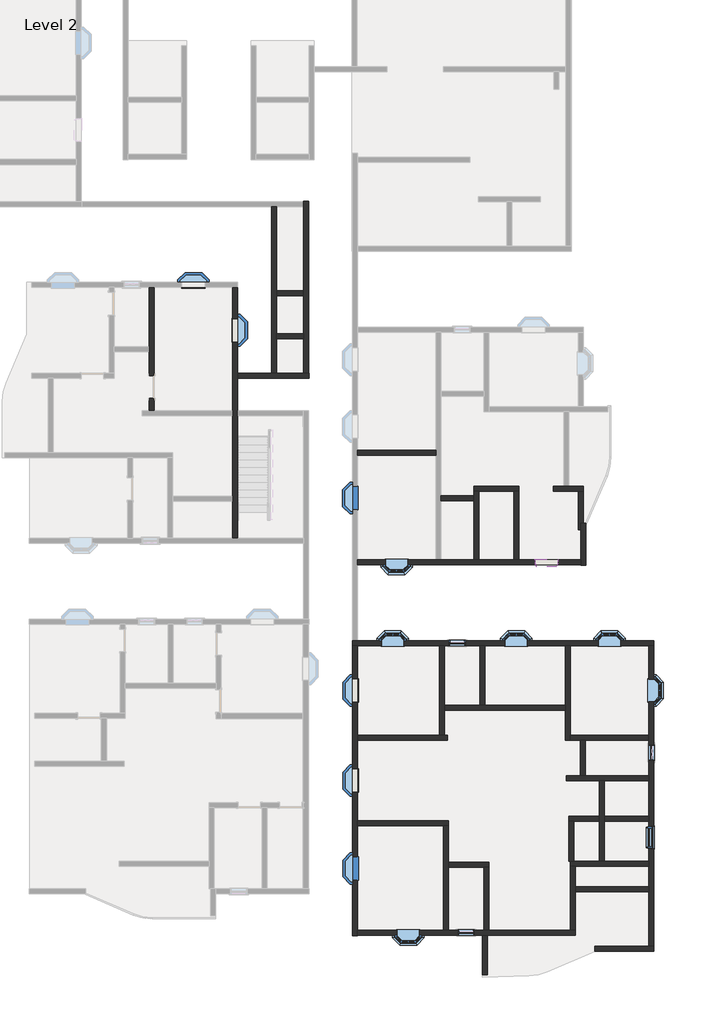
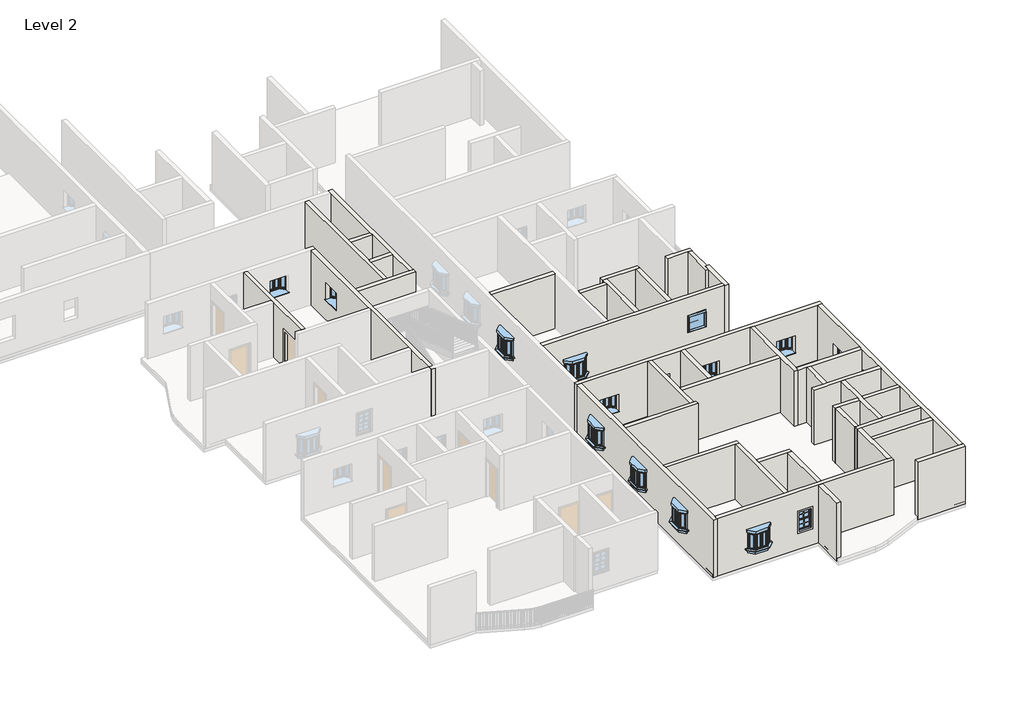
# One storey, part 2 of 14: 40 walls, 17 windows.
"""IFC4 building model written with IfcOpenShell, lengths in millimetres."""

from ifc_helpers import new_model, si_unit, frame, origin, place, context, project, spatial, polyline, outline, extrude, faceted_brep, transform, mapped, element, save
from components import window_910x910mm_67ef725a, window_8debb0fa, windows_sgl_w_glazing_bars_910x910mm_256712d0

model = new_model("IFC4")

# Units and contexts
model_context = context("Model", 3, world=origin())
ifc_project = project(units=[si_unit("LENGTHUNIT", "METRE", prefix="MILLI")], contexts=[model_context])

# Site, building, storey
site = spatial("IfcSite", under=ifc_project)
building = spatial("IfcBuilding", under=site)
storey = spatial("IfcBuildingStorey", under=building, Name="Level 2", Elevation=3048.0)

# Walls
placement = place(None, origin())
element("IfcWall", 1, ObjectType="4.5\" p", at=placement, inside=storey, context=model_context, shape_type="SweptSolid", body=[
    extrude(outline(polyline([(6070.4380523, -28382.7374148), (6070.4380523, -26796.6042694), (6273.6380523, -26796.6042694), (6273.6380523, -28382.7374148), (6070.4380523, -28382.7374148)])), frame((0.0, 0.0, 3048.0), z_axis=(0.0, 0.0, 1.0), x_axis=(1.0, 0.0, 0.0)), (0.0, 0.0, 1.0), 3048.0),
])
element("IfcWall", 2, ObjectType="4.5\" p", at=placement, inside=storey, context=model_context, shape_type="Brep", body=[
    faceted_brep([(10639.6896214, -27431.6042694, 3048.0), (13030.0380523, -27431.6042694, 3048.0), (13030.0380523, -27431.6042694, 6096.0), (10639.6896214, -27431.6042694, 6096.0), (10639.6896214, -27228.4042694, 3048.0), (10639.6896214, -27228.4042694, 6096.0), (12814.1380523, -27228.4042694, 6096.0), (13017.3380523, -27228.4042694, 6096.0), (13030.0380523, -27228.4042694, 6096.0), (13030.0380523, -27228.4042694, 3048.0), (13017.3380523, -27228.4042694, 3048.0), (12814.1380523, -27228.4042694, 3048.0)], [[[0, 1, 2, 3]], [[4, 5, 6, 7, 8, 9, 10, 11]], [[1, 0, 4, 11, 10, 9]], [[2, 1, 9, 8]], [[3, 2, 8, 7, 6, 5]], [[0, 3, 5, 4]]]),
])
element("IfcWall", 3, ObjectType="4.5\" p", at=placement, inside=storey, context=model_context, shape_type="Brep", body=[
    faceted_brep([(1015.8380523, -18878.1542694, 3048.0), (4648.0380523, -18878.1542694, 3048.0), (4648.0380523, -18878.1542694, 6096.0), (1015.8380523, -18878.1542694, 6096.0), (1015.8380523, -18674.9542694, 3048.0), (1015.8380523, -18674.9542694, 6096.0), (4336.8880523, -18674.9542694, 6096.0), (4540.0880523, -18674.9542694, 6096.0), (4648.0380523, -18674.9542694, 6096.0), (4648.0380523, -18674.9542694, 3048.0), (4540.0880523, -18674.9542694, 3048.0), (4336.8880523, -18674.9542694, 3048.0)], [[[0, 1, 2, 3]], [[4, 5, 6, 7, 8, 9, 10, 11]], [[1, 0, 4, 11, 10, 9]], [[2, 1, 9, 8]], [[3, 2, 8, 7, 6, 5]], [[0, 3, 5, 4]]]),
])
element("IfcWall", 4, ObjectType="4.5\" p", at=placement, inside=storey, context=model_context, shape_type="Brep", body=[
    faceted_brep([(4336.8880523, -15049.1042694, 3048.0), (4336.8880523, -18674.9542694, 3048.0), (4336.8880523, -18674.9542694, 6096.0), (4336.8880523, -15049.1042694, 6096.0), (4540.0880523, -15049.1042694, 3048.0), (4540.0880523, -15049.1042694, 6096.0), (4540.0880523, -17455.7542694, 6096.0), (4540.0880523, -17658.9542694, 6096.0), (4540.0880523, -18674.9542694, 6096.0), (4540.0880523, -18674.9542694, 3048.0), (4540.0880523, -17658.9542694, 3048.0), (4540.0880523, -17455.7542694, 3048.0)], [[[0, 1, 2, 3]], [[4, 5, 6, 7, 8, 9, 10, 11]], [[1, 0, 4, 11, 10, 9]], [[3, 2, 8, 7, 6, 5]], [[0, 3, 5, 4]], [[2, 1, 9, 8]]]),
])
element("IfcWall", 5, ObjectType="4.5\" p", at=placement, inside=storey, context=model_context, shape_type="Brep", body=[
    faceted_brep([(4540.0880523, -17658.9542694, 3048.0), (9442.2880523, -17658.9542694, 3048.0), (9442.2880523, -17658.9542694, 6096.0), (4540.0880523, -17658.9542694, 6096.0), (4540.0880523, -17455.7542694, 3048.0), (4540.0880523, -17455.7542694, 6096.0), (5975.1880523, -17455.7542694, 6096.0), (6178.3880523, -17455.7542694, 6096.0), (9442.2880523, -17455.7542694, 6096.0), (9442.2880523, -17455.7542694, 3048.0), (6178.3880523, -17455.7542694, 3048.0), (5975.1880523, -17455.7542694, 3048.0)], [[[0, 1, 2, 3]], [[4, 5, 6, 7, 8, 9, 10, 11]], [[1, 0, 4, 11, 10, 9]], [[3, 2, 8, 7, 6, 5]], [[0, 3, 5, 4]], [[2, 1, 9, 8]]]),
])
element("IfcWall", 6, ObjectType="4.5\" p", at=placement, inside=storey, context=model_context, shape_type="SweptSolid", body=[
    extrude(outline(polyline([(5975.1880523, -17455.7542694), (5975.1880523, -15049.1042694), (6178.3880523, -15049.1042694), (6178.3880523, -17455.7542694), (5975.1880523, -17455.7542694)])), frame((0.0, 0.0, 3048.0), z_axis=(0.0, 0.0, 1.0), x_axis=(1.0, 0.0, 0.0)), (0.0, 0.0, 1.0), 3048.0),
])
element("IfcWall", 7, ObjectType="4.5\" p", at=placement, inside=storey, context=model_context, shape_type="Brep", body=[
    faceted_brep([(9442.2880523, -15049.1042694, 3048.0), (9442.2880523, -17455.7542694, 3048.0), (9442.2880523, -17658.9542694, 3048.0), (9442.2880523, -18871.8042694, 3048.0), (9442.2880523, -18871.8042694, 6096.0), (9442.2880523, -17658.9542694, 6096.0), (9442.2880523, -17455.7542694, 6096.0), (9442.2880523, -15049.1042694, 6096.0), (9645.4880523, -15049.1042694, 3048.0), (9645.4880523, -15049.1042694, 6096.0), (9645.4880523, -18668.6042694, 6096.0), (9645.4880523, -18871.8042694, 6096.0), (9645.4880523, -18871.8042694, 3048.0), (9645.4880523, -18668.6042694, 3048.0)], [[[0, 1, 2, 3, 4, 5, 6, 7]], [[8, 9, 10, 11, 12, 13]], [[3, 2, 1, 0, 8, 13, 12]], [[7, 6, 5, 4, 11, 10, 9]], [[0, 7, 9, 8]], [[4, 3, 12, 11]]]),
])
element("IfcWall", 8, ObjectType="4.5\" p", at=placement, inside=storey, context=model_context, shape_type="Brep", body=[
    faceted_brep([(1015.8380523, -22345.2542694, 3048.0), (4489.2880523, -22345.2542694, 3048.0), (4692.4880523, -22345.2542694, 3048.0), (4692.4880523, -22345.2542694, 6096.0), (4489.2880523, -22345.2542694, 6096.0), (1015.8380523, -22345.2542694, 6096.0), (1015.8380523, -22142.0542694, 3048.0), (1015.8380523, -22142.0542694, 6096.0), (4692.4880523, -22142.0542694, 6096.0), (4692.4880523, -22142.0542694, 3048.0)], [[[0, 1, 2, 3, 4, 5]], [[6, 7, 8, 9]], [[2, 1, 0, 6, 9]], [[5, 4, 3, 8, 7]], [[0, 5, 7, 6]], [[3, 2, 9, 8]]]),
])
element("IfcWall", 9, ObjectType="4.5\" p", at=placement, inside=storey, context=model_context, shape_type="Brep", body=[
    faceted_brep([(4489.2880523, -22345.2542694, 3048.0), (4489.2880523, -26580.7042694, 3048.0), (4489.2880523, -26580.7042694, 6096.0), (4489.2880523, -22345.2542694, 6096.0), (4692.4880523, -22345.2542694, 3048.0), (4692.4880523, -22345.2542694, 6096.0), (4692.4880523, -23818.4542694, 6096.0), (4692.4880523, -24021.6542694, 6096.0), (4692.4880523, -26580.7042694, 6096.0), (4692.4880523, -26580.7042694, 3048.0), (4692.4880523, -24021.6542694, 3048.0), (4692.4880523, -23818.4542694, 3048.0)], [[[0, 1, 2, 3]], [[4, 5, 6, 7, 8, 9, 10, 11]], [[1, 0, 4, 11, 10, 9]], [[3, 2, 8, 7, 6, 5]], [[0, 3, 5, 4]], [[2, 1, 9, 8]]]),
])
element("IfcWall", 10, ObjectType="4.5\" p", at=placement, inside=storey, context=model_context, shape_type="Brep", body=[
    faceted_brep([(4692.4880523, -24021.6542694, 3048.0), (6127.5880523, -24021.6542694, 3048.0), (6330.7880523, -24021.6542694, 3048.0), (6330.7880523, -24021.6542694, 6096.0), (6127.5880523, -24021.6542694, 6096.0), (4692.4880523, -24021.6542694, 6096.0), (4692.4880523, -23818.4542694, 3048.0), (4692.4880523, -23818.4542694, 6096.0), (6330.7880523, -23818.4542694, 6096.0), (6330.7880523, -23818.4542694, 3048.0)], [[[0, 1, 2, 3, 4, 5]], [[6, 7, 8, 9]], [[2, 1, 0, 6, 9]], [[5, 4, 3, 8, 7]], [[0, 5, 7, 6]], [[3, 2, 9, 8]]]),
])
element("IfcWall", 11, ObjectType="4.5\" p", at=placement, inside=storey, context=model_context, shape_type="SweptSolid", body=[
    extrude(outline(polyline([(6127.5880523, -26580.7042694), (6127.5880523, -24021.6542694), (6330.7880523, -24021.6542694), (6330.7880523, -26580.7042694), (6127.5880523, -26580.7042694)])), frame((0.0, 0.0, 3048.0), z_axis=(0.0, 0.0, 1.0), x_axis=(1.0, 0.0, 0.0)), (0.0, 0.0, 1.0), 3048.0),
])
element("IfcWall", 12, ObjectType="4.5\" p", at=placement, inside=storey, context=model_context, shape_type="Brep", body=[
    faceted_brep([(9645.4880523, -18871.8042694, 3048.0), (10051.8880523, -18871.8042694, 3048.0), (10255.0880523, -18871.8042694, 3048.0), (12814.1380523, -18871.8042694, 3048.0), (12814.1380523, -18871.8042694, 6096.0), (10255.0880523, -18871.8042694, 6096.0), (10051.8880523, -18871.8042694, 6096.0), (9645.4880523, -18871.8042694, 6096.0), (9645.4880523, -18668.6042694, 3048.0), (9645.4880523, -18668.6042694, 6096.0), (12814.1380523, -18668.6042694, 6096.0), (12814.1380523, -18668.6042694, 3048.0)], [[[0, 1, 2, 3, 4, 5, 6, 7]], [[8, 9, 10, 11]], [[3, 2, 1, 0, 8, 11]], [[7, 6, 5, 4, 10, 9]], [[0, 7, 9, 8]], [[4, 3, 11, 10]]]),
])
element("IfcWall", 13, ObjectType="4.5\" p", at=placement, inside=storey, context=model_context, shape_type="SweptSolid", body=[
    extrude(outline(polyline([(10051.8880523, -20313.2542694), (10051.8880523, -18871.8042694), (10255.0880523, -18871.8042694), (10255.0880523, -20313.2542694), (10051.8880523, -20313.2542694)])), frame((0.0, 0.0, 3048.0), z_axis=(0.0, 0.0, 1.0), x_axis=(1.0, 0.0, 0.0)), (0.0, 0.0, 1.0), 3048.0),
])
element("IfcWall", 14, ObjectType="4.5\" p", at=placement, inside=storey, context=model_context, shape_type="Brep", body=[
    faceted_brep([(12814.1380523, -20313.2542694, 3048.0), (10255.0880523, -20313.2542694, 3048.0), (10051.8880523, -20313.2542694, 3048.0), (9486.7380523, -20313.2542694, 3048.0), (9486.7380523, -20313.2542694, 6096.0), (10051.8880523, -20313.2542694, 6096.0), (10255.0880523, -20313.2542694, 6096.0), (12814.1380523, -20313.2542694, 6096.0), (12814.1380523, -20516.4542694, 3048.0), (12814.1380523, -20516.4542694, 6096.0), (11017.0880523, -20516.4542694, 6096.0), (10813.8880523, -20516.4542694, 6096.0), (9486.7380523, -20516.4542694, 6096.0), (9486.7380523, -20516.4542694, 3048.0), (10813.8880523, -20516.4542694, 3048.0), (11017.0880523, -20516.4542694, 3048.0)], [[[0, 1, 2, 3, 4, 5, 6, 7]], [[8, 9, 10, 11, 12, 13, 14, 15]], [[3, 2, 1, 0, 8, 15, 14, 13]], [[4, 3, 13, 12]], [[7, 6, 5, 4, 12, 11, 10, 9]], [[0, 7, 9, 8]]]),
])
element("IfcWall", 15, ObjectType="4.5\" p", at=placement, inside=storey, context=model_context, shape_type="Brep", body=[
    faceted_brep([(10813.8880523, -20516.4542694, 3048.0), (10813.8880523, -21951.5542694, 3048.0), (10813.8880523, -22154.7542694, 3048.0), (10813.8880523, -23779.5416506, 3048.0), (10813.8880523, -23779.5416506, 6096.0), (10813.8880523, -22154.7542694, 6096.0), (10813.8880523, -21951.5542694, 6096.0), (10813.8880523, -20516.4542694, 6096.0), (11017.0880523, -20516.4542694, 3048.0), (11017.0880523, -20516.4542694, 6096.0), (11017.0880523, -21951.5542694, 6096.0), (11017.0880523, -22154.7542694, 6096.0), (11017.0880523, -23779.5416506, 6096.0), (11017.0880523, -23779.5416506, 3048.0), (11017.0880523, -22154.7542694, 3048.0), (11017.0880523, -21951.5542694, 3048.0)], [[[0, 1, 2, 3, 4, 5, 6, 7]], [[8, 9, 10, 11, 12, 13, 14, 15]], [[3, 2, 1, 0, 8, 15, 14, 13]], [[7, 6, 5, 4, 12, 11, 10, 9]], [[0, 7, 9, 8]], [[4, 3, 13, 12]]]),
])
element("IfcWall", 16, ObjectType="4.5\" p", at=placement, inside=storey, context=model_context, shape_type="Brep", body=[
    faceted_brep([(12814.1380523, -23779.5416506, 3048.0), (11017.0880523, -23779.5416506, 3048.0), (10813.8880523, -23779.5416506, 3048.0), (9791.5380523, -23779.5416506, 3048.0), (9632.7880523, -23779.5416506, 3048.0), (9632.7880523, -23779.5416506, 6096.0), (9791.5380523, -23779.5416506, 6096.0), (10813.8880523, -23779.5416506, 6096.0), (11017.0880523, -23779.5416506, 6096.0), (12814.1380523, -23779.5416506, 6096.0), (12814.1380523, -23982.7416506, 3048.0), (12814.1380523, -23982.7416506, 6096.0), (9835.9880523, -23982.7416506, 6096.0), (9632.7880523, -23982.7416506, 6096.0), (9632.7880523, -23982.7416506, 3048.0), (9835.9880523, -23982.7416506, 3048.0)], [[[0, 1, 2, 3, 4, 5, 6, 7, 8, 9]], [[10, 11, 12, 13, 14, 15]], [[4, 3, 2, 1, 0, 10, 15, 14]], [[9, 8, 7, 6, 5, 13, 12, 11]], [[0, 9, 11, 10]], [[5, 4, 14, 13]]]),
])
element("IfcWall", 17, ObjectType="4.5\" p", at=placement, inside=storey, context=model_context, shape_type="Brep", body=[
    faceted_brep([(9632.7880523, -23982.7416506, 3048.0), (9632.7880523, -26580.7042694, 3048.0), (9632.7880523, -26580.7042694, 6096.0), (9632.7880523, -23982.7416506, 6096.0), (9835.9880523, -23982.7416506, 3048.0), (9835.9880523, -23982.7416506, 6096.0), (9835.9880523, -24805.3496998, 6096.0), (9835.9880523, -25008.5496998, 6096.0), (9835.9880523, -26580.7042694, 6096.0), (9835.9880523, -26580.7042694, 3048.0), (9835.9880523, -25008.5496998, 3048.0), (9835.9880523, -24805.3496998, 3048.0)], [[[0, 1, 2, 3]], [[4, 5, 6, 7, 8, 9, 10, 11]], [[1, 0, 4, 11, 10, 9]], [[3, 2, 8, 7, 6, 5]], [[2, 1, 9, 8]], [[0, 3, 5, 4]]]),
])
element("IfcWall", 18, ObjectType="4.5\" p", at=placement, inside=storey, context=model_context, shape_type="SweptSolid", body=[
    extrude(outline(polyline([(12814.1380523, -25008.5496998), (9835.9880523, -25008.5496998), (9835.9880523, -24805.3496998), (12814.1380523, -24805.3496998), (12814.1380523, -25008.5496998)])), frame((0.0, 0.0, 3048.0), z_axis=(0.0, 0.0, 1.0), x_axis=(1.0, 0.0, 0.0)), (0.0, 0.0, 1.0), 3048.0),
])
element("IfcWall", 19, ObjectType="4.5\" p", at=placement, inside=storey, context=model_context, shape_type="Brep", body=[
    faceted_brep([(-7432.737215, -5015.2916506, 5181.6), (-7432.737215, -5015.2916506, 3048.0), (-7432.737215, -5523.2916506, 3048.0), (-7432.737215, -5523.2916506, 6096.0), (-7432.737215, -3135.6916506, 6096.0), (-7432.737215, -2932.4916506, 6096.0), (-7432.737215, -525.8416506, 6096.0), (-7432.737215, -525.8416506, 3048.0), (-7432.737215, -2932.4916506, 3048.0), (-7432.737215, -3135.6916506, 3048.0), (-7432.737215, -4100.8916506, 3048.0), (-7432.737215, -4100.8916506, 5181.6), (-7229.537215, -5523.2916506, 3048.0), (-7229.537215, -5015.2916506, 3048.0), (-7229.537215, -5015.2916506, 5181.6), (-7229.537215, -4100.8916506, 5181.6), (-7229.537215, -4100.8916506, 3048.0), (-7229.537215, -525.8416506, 3048.0), (-7229.537215, -525.8416506, 6096.0), (-7229.537215, -5523.2916506, 6096.0)], [[[0, 1, 2, 3, 4, 5, 6, 7, 8, 9, 10, 11]], [[12, 13, 14, 15, 16, 17, 18, 19]], [[2, 1, 13, 12]], [[10, 9, 8, 7, 17, 16]], [[6, 5, 4, 3, 19, 18]], [[7, 6, 18, 17]], [[3, 2, 12, 19]], [[14, 13, 1, 0]], [[15, 14, 0, 11]], [[16, 15, 11, 10]]]),
])
element("IfcWall", 20, ObjectType="4.5\" p", at=placement, inside=storey, context=model_context, shape_type="Brep", body=[
    faceted_brep([(-3857.687215, -4202.4916506, 3048.0), (-961.4891351, -4202.4916506, 3048.0), (-961.4891351, -4202.4916506, 6096.0), (-3857.687215, -4202.4916506, 6096.0), (-3857.687215, -3999.2916506, 3048.0), (-3857.687215, -3999.2916506, 6096.0), (-2472.7891351, -3999.2916506, 6096.0), (-2269.5891351, -3999.2916506, 6096.0), (-1177.3891351, -3999.2916506, 6096.0), (-974.1891351, -3999.2916506, 6096.0), (-961.4891351, -3999.2916506, 6096.0), (-961.4891351, -3999.2916506, 3048.0), (-974.1891351, -3999.2916506, 3048.0), (-1177.3891351, -3999.2916506, 3048.0), (-2269.5891351, -3999.2916506, 3048.0), (-2472.7891351, -3999.2916506, 3048.0)], [[[0, 1, 2, 3]], [[4, 5, 6, 7, 8, 9, 10, 11, 12, 13, 14, 15]], [[1, 0, 4, 15, 14, 13, 12, 11]], [[2, 1, 11, 10]], [[3, 2, 10, 9, 8, 7, 6, 5]], [[0, 3, 5, 4]]]),
])
element("IfcWall", 21, ObjectType="4.5\" p", at=placement, inside=storey, context=model_context, shape_type="SweptSolid", body=[
    extrude(outline(polyline([(-1177.3891351, -868.7416506), (-2269.5891351, -868.7416506), (-2269.5891351, -665.5416506), (-1177.3891351, -665.5416506), (-1177.3891351, -868.7416506)])), frame((0.0, 0.0, 3048.0), z_axis=(0.0, 0.0, 1.0), x_axis=(1.0, 0.0, 0.0)), (0.0, 0.0, 1.0), 3048.0),
])
element("IfcWall", 22, ObjectType="4.5\" p", at=placement, inside=storey, context=model_context, shape_type="SweptSolid", body=[
    extrude(outline(polyline([(-1177.3891351, -2597.8466506), (-2269.5891351, -2597.8466506), (-2269.5891351, -2394.6466506), (-1177.3891351, -2394.6466506), (-1177.3891351, -2597.8466506)])), frame((0.0, 0.0, 3048.0), z_axis=(0.0, 0.0, 1.0), x_axis=(1.0, 0.0, 0.0)), (0.0, 0.0, 1.0), 3048.0),
])
element("IfcWall", 23, ObjectType="4.5\" p", at=placement, inside=storey, context=model_context, shape_type="SweptSolid", body=[
    extrude(outline(polyline([(5721.1880523, -9162.6542694), (4387.6880523, -9162.6542694), (4387.6880523, -8959.4542694), (5721.1880523, -8959.4542694), (5721.1880523, -9162.6542694)])), frame((0.0, 0.0, 3048.0), z_axis=(0.0, 0.0, 1.0), x_axis=(1.0, 0.0, 0.0)), (0.0, 0.0, 1.0), 3048.0),
])
element("IfcWall", 24, ObjectType="4.5\" p", at=placement, inside=storey, context=model_context, shape_type="Brep", body=[
    faceted_brep([(5721.1880523, -8781.6542694, 3048.0), (5924.3880523, -8781.6542694, 3048.0), (7359.4880523, -8781.6542694, 3048.0), (7562.6880523, -8781.6542694, 3048.0), (7562.6880523, -8781.6542694, 6096.0), (7359.4880523, -8781.6542694, 6096.0), (5924.3880523, -8781.6542694, 6096.0), (5721.1880523, -8781.6542694, 6096.0), (5721.1880523, -8578.4542694, 3048.0), (5721.1880523, -8578.4542694, 6096.0), (7562.6880523, -8578.4542694, 6096.0), (7562.6880523, -8578.4542694, 3048.0)], [[[0, 1, 2, 3, 4, 5, 6, 7]], [[8, 9, 10, 11]], [[3, 2, 1, 0, 8, 11]], [[7, 6, 5, 4, 10, 9]], [[0, 7, 9, 8]], [[4, 3, 11, 10]]]),
])
element("IfcWall", 25, ObjectType="4.5\" p", at=placement, inside=storey, context=model_context, shape_type="Brep", body=[
    faceted_brep([(5721.1880523, -8781.6542694, 3048.0), (5721.1880523, -8959.4542694, 3048.0), (5721.1880523, -9162.6542694, 3048.0), (5721.1880523, -11556.6042694, 3048.0), (5721.1880523, -11556.6042694, 6096.0), (5721.1880523, -9162.6542694, 6096.0), (5721.1880523, -8959.4542694, 6096.0), (5721.1880523, -8781.6542694, 6096.0), (5924.3880523, -8781.6542694, 3048.0), (5924.3880523, -8781.6542694, 6096.0), (5924.3880523, -11556.6042694, 6096.0), (5924.3880523, -11556.6042694, 3048.0)], [[[0, 1, 2, 3, 4, 5, 6, 7]], [[8, 9, 10, 11]], [[3, 2, 1, 0, 8, 11]], [[7, 6, 5, 4, 10, 9]], [[0, 7, 9, 8]], [[4, 3, 11, 10]]]),
])
element("IfcWall", 26, ObjectType="4.5\" p", at=placement, inside=storey, context=model_context, shape_type="SweptSolid", body=[
    extrude(outline(polyline([(7359.4880523, -11556.6042694), (7359.4880523, -8781.6542694), (7562.6880523, -8781.6542694), (7562.6880523, -11556.6042694), (7359.4880523, -11556.6042694)])), frame((0.0, 0.0, 3048.0), z_axis=(0.0, 0.0, 1.0), x_axis=(1.0, 0.0, 0.0)), (0.0, 0.0, 1.0), 3048.0),
])
element("IfcWall", 27, ObjectType="4.5\" p", at=placement, inside=storey, context=model_context, shape_type="SweptSolid", body=[
    extrude(outline(polyline([(4184.4880523, -7333.8542694), (1007.0108649, -7333.8542694), (1007.0108649, -7130.6542694), (4184.4880523, -7130.6542694), (4184.4880523, -7333.8542694)])), frame((0.0, 0.0, 3048.0), z_axis=(0.0, 0.0, 1.0), x_axis=(1.0, 0.0, 0.0)), (0.0, 0.0, 1.0), 3048.0),
])
element("IfcWall", 28, ObjectType="4.5\" p", at=placement, inside=storey, context=model_context, shape_type="Brep", body=[
    faceted_brep([(8953.3380523, -8781.6542694, 3048.0), (9956.6380523, -8781.6542694, 3048.0), (10159.8380523, -8781.6542694, 3048.0), (10172.5380523, -8781.6542694, 3048.0), (10172.5380523, -8781.6542694, 6096.0), (10159.8380523, -8781.6542694, 6096.0), (9956.6380523, -8781.6542694, 6096.0), (8953.3380523, -8781.6542694, 6096.0), (8953.3380523, -8578.4542694, 3048.0), (8953.3380523, -8578.4542694, 6096.0), (9371.2322031, -8578.4542694, 6096.0), (9574.4322031, -8578.4542694, 6096.0), (10172.5380523, -8578.4542694, 6096.0), (10172.5380523, -8578.4542694, 3048.0), (9574.4322031, -8578.4542694, 3048.0), (9371.2322031, -8578.4542694, 3048.0)], [[[0, 1, 2, 3, 4, 5, 6, 7]], [[8, 9, 10, 11, 12, 13, 14, 15]], [[3, 2, 1, 0, 8, 15, 14, 13]], [[4, 3, 13, 12]], [[7, 6, 5, 4, 12, 11, 10, 9]], [[0, 7, 9, 8]]]),
])
element("IfcWall", 29, ObjectType="4.5\" p", at=placement, inside=storey, context=model_context, shape_type="SweptSolid", body=[
    extrude(outline(polyline([(9956.6380523, -10352.8912671), (9956.6380523, -8781.6542694), (10159.8380523, -8781.6542694), (10159.8380523, -10352.8912671), (9956.6380523, -10352.8912671)])), frame((0.0, 0.0, 3048.0), z_axis=(0.0, 0.0, 1.0), x_axis=(1.0, 0.0, 0.0)), (0.0, 0.0, 1.0), 3048.0),
])
element("IfcWall", 30, ObjectType="4.5\" p", at=placement, inside=storey, context=model_context, shape_type="Brep", body=[
    faceted_brep([(12814.1380523, -21951.5542694, 6096.0), (12814.1380523, -21951.5542694, 3048.0), (11017.0880523, -21951.5542694, 3048.0), (11017.0880523, -21951.5542694, 6096.0), (12814.1380523, -22154.7542694, 3048.0), (12814.1380523, -22154.7542694, 6096.0), (11017.0880523, -22154.7542694, 6096.0), (11017.0880523, -22154.7542694, 3048.0)], [[[0, 1, 2, 3]], [[4, 5, 6, 7]], [[1, 4, 7, 2]], [[5, 0, 3, 6]], [[1, 0, 5, 4]], [[3, 2, 7, 6]]]),
    faceted_brep([(9588.3380523, -21951.5542694, 3048.0), (9588.3380523, -21951.5542694, 6096.0), (10813.8880523, -21951.5542694, 6096.0), (10813.8880523, -21951.5542694, 3048.0), (9588.3380523, -22154.7542694, 6096.0), (9588.3380523, -22154.7542694, 3048.0), (9791.5380523, -22154.7542694, 3048.0), (10813.8880523, -22154.7542694, 3048.0), (10813.8880523, -22154.7542694, 6096.0), (9791.5380523, -22154.7542694, 6096.0)], [[[0, 1, 2, 3]], [[4, 5, 6, 7, 8, 9]], [[5, 0, 3, 7, 6]], [[1, 4, 9, 8, 2]], [[3, 2, 8, 7]], [[1, 0, 5, 4]]]),
])
element("IfcWall", 31, ObjectType="4.5\" p", at=placement, inside=storey, context=model_context, shape_type="Brep", body=[
    faceted_brep([(9588.3380523, -22154.7542694, 3048.0), (9588.3380523, -23779.5416506, 3048.0), (9588.3380523, -23779.5416506, 6096.0), (9588.3380523, -22154.7542694, 6096.0), (9791.5380523, -22154.7542694, 3048.0), (9791.5380523, -22154.7542694, 6096.0), (9791.5380523, -23779.5416506, 6096.0), (9791.5380523, -23779.5416506, 3048.0), (9632.7880523, -23779.5416506, 3048.0), (9632.7880523, -23779.5416506, 6096.0)], [[[0, 1, 2, 3]], [[4, 5, 6, 7]], [[1, 0, 4, 7, 8]], [[3, 2, 9, 6, 5]], [[2, 1, 8, 7, 6, 9]], [[0, 3, 5, 4]]]),
])
element("IfcWall", 32, ObjectType="9\"", at=placement, inside=storey, context=model_context, shape_type="Brep", body=[
    faceted_brep([(799.9380523, -15049.1042694, 3048.0), (812.6380523, -15049.1042694, 3048.0), (1015.8380523, -15049.1042694, 3048.0), (4336.8880523, -15049.1042694, 3048.0), (4540.0880523, -15049.1042694, 3048.0), (5975.1880523, -15049.1042694, 3048.0), (6178.3880523, -15049.1042694, 3048.0), (9442.2880523, -15049.1042694, 3048.0), (9645.4880523, -15049.1042694, 3048.0), (12814.1380523, -15049.1042694, 3048.0), (13017.3380523, -15049.1042694, 3048.0), (13030.0380523, -15049.1042694, 3048.0), (13030.0380523, -15049.1042694, 6096.0), (13017.3380523, -15049.1042694, 6096.0), (12814.1380523, -15049.1042694, 6096.0), (9645.4880523, -15049.1042694, 6096.0), (9442.2880523, -15049.1042694, 6096.0), (6178.3880523, -15049.1042694, 6096.0), (5975.1880523, -15049.1042694, 6096.0), (4540.0880523, -15049.1042694, 6096.0), (4336.8880523, -15049.1042694, 6096.0), (1015.8380523, -15049.1042694, 6096.0), (812.6380523, -15049.1042694, 6096.0), (799.9380523, -15049.1042694, 6096.0), (1983.2380523, -15049.1042694, 4872.4), (2893.2380523, -15049.1042694, 4872.4), (2893.2380523, -15049.1042694, 3962.4), (1983.2380523, -15049.1042694, 3962.4), (10774.8130523, -15049.1042694, 4872.4), (11684.8130523, -15049.1042694, 4872.4), (11684.8130523, -15049.1042694, 3962.4), (10774.8130523, -15049.1042694, 3962.4), (6993.3880523, -15049.1042694, 4872.4), (7903.3880523, -15049.1042694, 4872.4), (7903.3880523, -15049.1042694, 3962.4), (6993.3880523, -15049.1042694, 3962.4), (4717.8880523, -15049.1042694, 5029.2), (5378.2880523, -15049.1042694, 5029.2), (5378.2880523, -15049.1042694, 3962.4), (4717.8880523, -15049.1042694, 3962.4), (799.9380523, -14845.9042694, 3048.0), (799.9380523, -14845.9042694, 6096.0), (803.8108649, -14845.9042694, 6096.0), (1007.0108649, -14845.9042694, 6096.0), (13030.0380523, -14845.9042694, 6096.0), (13030.0380523, -14845.9042694, 3048.0), (1007.0108649, -14845.9042694, 3048.0), (803.8108649, -14845.9042694, 3048.0), (1983.2380523, -14845.9042694, 4872.4), (1983.2380523, -14845.9042694, 3962.4), (2893.2380523, -14845.9042694, 3962.4), (2893.2380523, -14845.9042694, 4872.4), (10774.8130523, -14845.9042694, 4872.4), (10774.8130523, -14845.9042694, 3962.4), (11684.8130523, -14845.9042694, 3962.4), (11684.8130523, -14845.9042694, 4872.4), (6993.3880523, -14845.9042694, 4872.4), (6993.3880523, -14845.9042694, 3962.4), (7903.3880523, -14845.9042694, 3962.4), (7903.3880523, -14845.9042694, 4872.4), (4717.8880523, -14845.9042694, 5029.2), (4717.8880523, -14845.9042694, 3962.4), (5378.2880523, -14845.9042694, 3962.4), (5378.2880523, -14845.9042694, 5029.2)], [[[0, 1, 2, 3, 4, 5, 6, 7, 8, 9, 10, 11, 12, 13, 14, 15, 16, 17, 18, 19, 20, 21, 22, 23], [24, 25, 26, 27], [28, 29, 30, 31], [32, 33, 34, 35], [36, 37, 38, 39]], [[40, 41, 42, 43, 44, 45, 46, 47], [48, 49, 50, 51], [52, 53, 54, 55], [56, 57, 58, 59], [60, 61, 62, 63]], [[11, 10, 9, 8, 7, 6, 5, 4, 3, 2, 1, 0, 40, 47, 46, 45]], [[12, 11, 45, 44]], [[23, 22, 21, 20, 19, 18, 17, 16, 15, 14, 13, 12, 44, 43, 42, 41]], [[0, 23, 41, 40]], [[49, 48, 24, 27]], [[50, 49, 27, 26]], [[51, 50, 26, 25]], [[48, 51, 25, 24]], [[53, 52, 28, 31]], [[54, 53, 31, 30]], [[55, 54, 30, 29]], [[52, 55, 29, 28]], [[57, 56, 32, 35]], [[58, 57, 35, 34]], [[59, 58, 34, 33]], [[56, 59, 33, 32]], [[61, 60, 36, 39]], [[62, 61, 39, 38]], [[63, 62, 38, 37]], [[60, 63, 37, 36]]]),
])
element("IfcWall", 33, ObjectType="9\"", at=placement, inside=storey, context=model_context, shape_type="Brep", body=[
    faceted_brep([(12814.1380523, -15049.1042694, 3048.0), (12814.1380523, -18668.6042694, 3048.0), (12814.1380523, -18871.8042694, 3048.0), (12814.1380523, -20313.2542694, 3048.0), (12814.1380523, -20516.4542694, 3048.0), (12814.1380523, -21951.5542694, 3048.0), (12814.1380523, -22154.7542694, 3048.0), (12814.1380523, -23779.5416506, 3048.0), (12814.1380523, -23982.7416506, 3048.0), (12814.1380523, -24805.3496998, 3048.0), (12814.1380523, -25008.5496998, 3048.0), (12814.1380523, -27228.4042694, 3048.0), (12814.1380523, -27228.4042694, 6096.0), (12814.1380523, -25008.5496998, 6096.0), (12814.1380523, -24805.3496998, 6096.0), (12814.1380523, -23982.7416506, 6096.0), (12814.1380523, -23779.5416506, 6096.0), (12814.1380523, -22154.7542694, 6096.0), (12814.1380523, -21951.5542694, 6096.0), (12814.1380523, -20516.4542694, 6096.0), (12814.1380523, -20313.2542694, 6096.0), (12814.1380523, -18871.8042694, 6096.0), (12814.1380523, -18668.6042694, 6096.0), (12814.1380523, -15049.1042694, 6096.0), (12814.1380523, -16403.8542694, 4872.4), (12814.1380523, -17313.8542694, 4872.4), (12814.1380523, -17313.8542694, 3962.4), (12814.1380523, -16403.8542694, 3962.4), (12814.1380523, -23270.1542694, 4872.4), (12814.1380523, -23270.1542694, 3962.4), (12814.1380523, -22360.1542694, 3962.4), (12814.1380523, -22360.1542694, 4872.4), (12814.1380523, -19049.6042694, 5029.2), (12814.1380523, -19710.0042694, 5029.2), (12814.1380523, -19710.0042694, 3962.4), (12814.1380523, -19049.6042694, 3962.4), (13017.3380523, -15049.1042694, 3048.0), (13017.3380523, -15049.1042694, 6096.0), (13017.3380523, -27228.4042694, 6096.0), (13017.3380523, -27228.4042694, 3048.0), (13017.3380523, -16403.8542694, 4872.4), (13017.3380523, -16403.8542694, 3962.4), (13017.3380523, -17313.8542694, 3962.4), (13017.3380523, -17313.8542694, 4872.4), (13017.3380523, -23270.1542694, 4872.4), (13017.3380523, -22360.1542694, 4872.4), (13017.3380523, -22360.1542694, 3962.4), (13017.3380523, -23270.1542694, 3962.4), (13017.3380523, -19049.6042694, 5029.2), (13017.3380523, -19049.6042694, 3962.4), (13017.3380523, -19710.0042694, 3962.4), (13017.3380523, -19710.0042694, 5029.2)], [[[0, 1, 2, 3, 4, 5, 6, 7, 8, 9, 10, 11, 12, 13, 14, 15, 16, 17, 18, 19, 20, 21, 22, 23], [24, 25, 26, 27], [28, 29, 30, 31], [32, 33, 34, 35]], [[36, 37, 38, 39], [40, 41, 42, 43], [44, 45, 46, 47], [48, 49, 50, 51]], [[11, 10, 9, 8, 7, 6, 5, 4, 3, 2, 1, 0, 36, 39]], [[23, 22, 21, 20, 19, 18, 17, 16, 15, 14, 13, 12, 38, 37]], [[0, 23, 37, 36]], [[12, 11, 39, 38]], [[41, 40, 24, 27]], [[42, 41, 27, 26]], [[43, 42, 26, 25]], [[40, 43, 25, 24]], [[29, 28, 44, 47]], [[30, 29, 47, 46]], [[31, 30, 46, 45]], [[28, 31, 45, 44]], [[49, 48, 32, 35]], [[50, 49, 35, 34]], [[51, 50, 34, 33]], [[48, 51, 33, 32]]]),
])
element("IfcWall", 34, ObjectType="9\"", at=placement, inside=storey, context=model_context, shape_type="Brep", body=[
    faceted_brep([(812.6380523, -15049.1042694, 3048.0), (812.6380523, -26796.6042694, 3048.0), (812.6380523, -26796.6042694, 6096.0), (812.6380523, -15049.1042694, 6096.0), (812.6380523, -24527.4542694, 5158.0), (812.6380523, -24527.4542694, 4248.0), (812.6380523, -23617.4542694, 4248.0), (812.6380523, -23617.4542694, 5158.0), (812.6380523, -20965.1042694, 5158.0), (812.6380523, -20965.1042694, 4248.0), (812.6380523, -20055.1042694, 4248.0), (812.6380523, -20055.1042694, 5158.0), (812.6380523, -17317.0292694, 5158.0), (812.6380523, -17317.0292694, 4248.0), (812.6380523, -16407.0292694, 4248.0), (812.6380523, -16407.0292694, 5158.0), (1015.8380523, -15049.1042694, 3048.0), (1015.8380523, -15049.1042694, 6096.0), (1015.8380523, -18674.9542694, 6096.0), (1015.8380523, -18878.1542694, 6096.0), (1015.8380523, -22142.0542694, 6096.0), (1015.8380523, -22345.2542694, 6096.0), (1015.8380523, -26580.7042694, 6096.0), (1015.8380523, -26783.9042694, 6096.0), (1015.8380523, -26796.6042694, 6096.0), (1015.8380523, -26796.6042694, 3048.0), (1015.8380523, -26783.9042694, 3048.0), (1015.8380523, -26580.7042694, 3048.0), (1015.8380523, -22345.2542694, 3048.0), (1015.8380523, -22142.0542694, 3048.0), (1015.8380523, -18878.1542694, 3048.0), (1015.8380523, -18674.9542694, 3048.0), (1015.8380523, -24527.4542694, 5158.0), (1015.8380523, -23617.4542694, 5158.0), (1015.8380523, -23617.4542694, 4248.0), (1015.8380523, -24527.4542694, 4248.0), (1015.8380523, -20965.1042694, 5158.0), (1015.8380523, -20055.1042694, 5158.0), (1015.8380523, -20055.1042694, 4248.0), (1015.8380523, -20965.1042694, 4248.0), (1015.8380523, -17317.0292694, 5158.0), (1015.8380523, -16407.0292694, 5158.0), (1015.8380523, -16407.0292694, 4248.0), (1015.8380523, -17317.0292694, 4248.0)], [[[0, 1, 2, 3], [4, 5, 6, 7], [8, 9, 10, 11], [12, 13, 14, 15]], [[16, 17, 18, 19, 20, 21, 22, 23, 24, 25, 26, 27, 28, 29, 30, 31], [32, 33, 34, 35], [36, 37, 38, 39], [40, 41, 42, 43]], [[1, 0, 16, 31, 30, 29, 28, 27, 26, 25]], [[2, 1, 25, 24]], [[3, 2, 24, 23, 22, 21, 20, 19, 18, 17]], [[0, 3, 17, 16]], [[5, 4, 32, 35]], [[6, 5, 35, 34]], [[7, 6, 34, 33]], [[4, 7, 33, 32]], [[9, 8, 36, 39]], [[10, 9, 39, 38]], [[11, 10, 38, 37]], [[8, 11, 37, 36]], [[13, 12, 40, 43]], [[14, 13, 43, 42]], [[15, 14, 42, 41]], [[12, 15, 41, 40]]]),
])
element("IfcWall", 35, ObjectType="9\"", at=placement, inside=storey, context=model_context, shape_type="Brep", body=[
    faceted_brep([(1015.8380523, -26783.9042694, 3048.0), (9835.9880523, -26783.9042694, 3048.0), (9835.9880523, -26783.9042694, 6096.0), (1015.8380523, -26783.9042694, 6096.0), (3521.8880523, -26783.9042694, 4872.4), (3521.8880523, -26783.9042694, 3962.4), (2611.8880523, -26783.9042694, 3962.4), (2611.8880523, -26783.9042694, 4872.4), (5079.8380523, -26783.9042694, 5029.2), (5740.2380523, -26783.9042694, 5029.2), (5740.2380523, -26783.9042694, 3962.4), (5079.8380523, -26783.9042694, 3962.4), (1015.8380523, -26580.7042694, 3048.0), (1015.8380523, -26580.7042694, 6096.0), (4489.2880523, -26580.7042694, 6096.0), (4692.4880523, -26580.7042694, 6096.0), (6127.5880523, -26580.7042694, 6096.0), (6330.7880523, -26580.7042694, 6096.0), (9632.7880523, -26580.7042694, 6096.0), (9835.9880523, -26580.7042694, 6096.0), (9835.9880523, -26580.7042694, 3048.0), (9632.7880523, -26580.7042694, 3048.0), (6330.7880523, -26580.7042694, 3048.0), (6127.5880523, -26580.7042694, 3048.0), (4692.4880523, -26580.7042694, 3048.0), (4489.2880523, -26580.7042694, 3048.0), (3521.8880523, -26580.7042694, 4872.4), (2611.8880523, -26580.7042694, 4872.4), (2611.8880523, -26580.7042694, 3962.4), (3521.8880523, -26580.7042694, 3962.4), (5079.8380523, -26580.7042694, 5029.2), (5079.8380523, -26580.7042694, 3962.4), (5740.2380523, -26580.7042694, 3962.4), (5740.2380523, -26580.7042694, 5029.2)], [[[0, 1, 2, 3], [4, 5, 6, 7], [8, 9, 10, 11]], [[12, 13, 14, 15, 16, 17, 18, 19, 20, 21, 22, 23, 24, 25], [26, 27, 28, 29], [30, 31, 32, 33]], [[1, 0, 12, 25, 24, 23, 22, 21, 20]], [[3, 2, 19, 18, 17, 16, 15, 14, 13]], [[0, 3, 13, 12]], [[2, 1, 20, 19]], [[5, 4, 26, 29]], [[6, 5, 29, 28]], [[7, 6, 28, 27]], [[4, 7, 27, 26]], [[31, 30, 8, 11]], [[32, 31, 11, 10]], [[33, 32, 10, 9]], [[30, 33, 9, 8]]]),
])
element("IfcWall", 36, ObjectType="9\" w", at=placement, inside=storey, context=model_context, shape_type="Brep", body=[
    faceted_brep([(-4060.887215, -525.8416506, 3048.0), (-4060.887215, -5523.2916506, 3048.0), (-4060.887215, -5726.4916506, 3048.0), (-4060.887215, -8990.3916506, 3048.0), (-4060.887215, -9193.5916506, 3048.0), (-4060.887215, -10901.7416506, 3048.0), (-4060.887215, -10901.7416506, 6096.0), (-4060.887215, -9193.5916506, 6096.0), (-4060.887215, -8990.3916506, 6096.0), (-4060.887215, -5726.4916506, 6096.0), (-4060.887215, -5523.2916506, 6096.0), (-4060.887215, -525.8416506, 6096.0), (-4060.887215, -1807.5666506, 5158.0), (-4060.887215, -2717.5666506, 5158.0), (-4060.887215, -2717.5666506, 4248.0), (-4060.887215, -1807.5666506, 4248.0), (-3857.687215, -525.8416506, 3048.0), (-3857.687215, -525.8416506, 6096.0), (-3857.687215, -3999.2916506, 6096.0), (-3857.687215, -4202.4916506, 6096.0), (-3857.687215, -5523.2916506, 6096.0), (-3857.687215, -5726.4916506, 6096.0), (-3857.687215, -10901.7416506, 6096.0), (-3857.687215, -10901.7416506, 3048.0), (-3857.687215, -5726.4916506, 3048.0), (-3857.687215, -5523.2916506, 3048.0), (-3857.687215, -4202.4916506, 3048.0), (-3857.687215, -3999.2916506, 3048.0), (-3857.687215, -1807.5666506, 5158.0), (-3857.687215, -1807.5666506, 4248.0), (-3857.687215, -2717.5666506, 4248.0), (-3857.687215, -2717.5666506, 5158.0)], [[[0, 1, 2, 3, 4, 5, 6, 7, 8, 9, 10, 11], [12, 13, 14, 15]], [[16, 17, 18, 19, 20, 21, 22, 23, 24, 25, 26, 27], [28, 29, 30, 31]], [[5, 4, 3, 2, 1, 0, 16, 27, 26, 25, 24, 23]], [[6, 5, 23, 22]], [[11, 10, 9, 8, 7, 6, 22, 21, 20, 19, 18, 17]], [[0, 11, 17, 16]], [[29, 28, 12, 15]], [[30, 29, 15, 14]], [[31, 30, 14, 13]], [[28, 31, 13, 12]]]),
])
element("IfcWall", 37, ObjectType="9\" w", at=placement, inside=storey, context=model_context, shape_type="Brep", body=[
    faceted_brep([(-2269.5891351, -3999.2916506, 3048.0), (-2269.5891351, -2597.8466506, 3048.0), (-2269.5891351, -2394.6466506, 3048.0), (-2269.5891351, -868.7416506, 3048.0), (-2269.5891351, -665.5416506, 3048.0), (-2269.5891351, 2750.7583494, 3048.0), (-2269.5891351, 2750.7583494, 6096.0), (-2269.5891351, -665.5416506, 6096.0), (-2269.5891351, -868.7416506, 6096.0), (-2269.5891351, -2394.6466506, 6096.0), (-2269.5891351, -2597.8466506, 6096.0), (-2269.5891351, -3999.2916506, 6096.0), (-2472.7891351, -3999.2916506, 3048.0), (-2472.7891351, -3999.2916506, 6096.0), (-2472.7891351, 2750.7583494, 6096.0), (-2472.7891351, 2750.7583494, 3048.0)], [[[0, 1, 2, 3, 4, 5, 6, 7, 8, 9, 10, 11]], [[12, 13, 14, 15]], [[5, 4, 3, 2, 1, 0, 12, 15]], [[11, 10, 9, 8, 7, 6, 14, 13]], [[0, 11, 13, 12]], [[6, 5, 15, 14]]]),
])
element("IfcWall", 38, ObjectType="9\" w", at=placement, inside=storey, context=model_context, shape_type="Brep", body=[
    faceted_brep([(-974.1891351, -3999.2916506, 3048.0), (-974.1891351, 2966.6583494, 3048.0), (-974.1891351, 2966.6583494, 6096.0), (-974.1891351, -3999.2916506, 6096.0), (-1177.3891351, -3999.2916506, 3048.0), (-1177.3891351, -3999.2916506, 6096.0), (-1177.3891351, -2597.8466506, 6096.0), (-1177.3891351, -2394.6466506, 6096.0), (-1177.3891351, -868.7416506, 6096.0), (-1177.3891351, -665.5416506, 6096.0), (-1177.3891351, 2750.7583494, 6096.0), (-1177.3891351, 2953.9583494, 6096.0), (-1177.3891351, 2966.6583494, 6096.0), (-1177.3891351, 2966.6583494, 3048.0), (-1177.3891351, 2953.9583494, 3048.0), (-1177.3891351, 2750.7583494, 3048.0), (-1177.3891351, -665.5416506, 3048.0), (-1177.3891351, -868.7416506, 3048.0), (-1177.3891351, -2394.6466506, 3048.0), (-1177.3891351, -2597.8466506, 3048.0)], [[[0, 1, 2, 3]], [[4, 5, 6, 7, 8, 9, 10, 11, 12, 13, 14, 15, 16, 17, 18, 19]], [[1, 0, 4, 19, 18, 17, 16, 15, 14, 13]], [[2, 1, 13, 12]], [[3, 2, 12, 11, 10, 9, 8, 7, 6, 5]], [[0, 3, 5, 4]]]),
])
element("IfcWall", 39, ObjectType="9\" w", at=placement, inside=storey, context=model_context, shape_type="Brep", body=[
    faceted_brep([(1007.0108649, -11759.8042694, 3048.0), (10070.9380523, -11759.8042694, 3048.0), (10070.9380523, -11759.8042694, 6096.0), (1007.0108649, -11759.8042694, 6096.0), (3050.7494586, -11759.8042694, 4872.4), (3050.7494586, -11759.8042694, 3962.4), (2140.7494586, -11759.8042694, 3962.4), (2140.7494586, -11759.8042694, 4872.4), (9135.2880523, -11759.8042694, 5158.0), (9135.2880523, -11759.8042694, 4248.0), (8225.2880523, -11759.8042694, 4248.0), (8225.2880523, -11759.8042694, 5158.0), (1007.0108649, -11556.6042694, 3048.0), (1007.0108649, -11556.6042694, 6096.0), (4184.4880523, -11556.6042694, 6096.0), (4387.6880523, -11556.6042694, 6096.0), (5721.1880523, -11556.6042694, 6096.0), (5924.3880523, -11556.6042694, 6096.0), (7359.4880523, -11556.6042694, 6096.0), (7562.6880523, -11556.6042694, 6096.0), (10070.9380523, -11556.6042694, 6096.0), (10070.9380523, -11556.6042694, 3048.0), (7562.6880523, -11556.6042694, 3048.0), (7359.4880523, -11556.6042694, 3048.0), (5924.3880523, -11556.6042694, 3048.0), (5721.1880523, -11556.6042694, 3048.0), (4387.6880523, -11556.6042694, 3048.0), (4184.4880523, -11556.6042694, 3048.0), (3050.7494586, -11556.6042694, 4872.4), (2140.7494586, -11556.6042694, 4872.4), (2140.7494586, -11556.6042694, 3962.4), (3050.7494586, -11556.6042694, 3962.4), (9135.2880523, -11556.6042694, 5158.0), (8225.2880523, -11556.6042694, 5158.0), (8225.2880523, -11556.6042694, 4248.0), (9135.2880523, -11556.6042694, 4248.0)], [[[0, 1, 2, 3], [4, 5, 6, 7], [8, 9, 10, 11]], [[12, 13, 14, 15, 16, 17, 18, 19, 20, 21, 22, 23, 24, 25, 26, 27], [28, 29, 30, 31], [32, 33, 34, 35]], [[1, 0, 12, 27, 26, 25, 24, 23, 22, 21]], [[3, 2, 20, 19, 18, 17, 16, 15, 14, 13]], [[0, 3, 13, 12]], [[2, 1, 21, 20]], [[5, 4, 28, 31]], [[6, 5, 31, 30]], [[7, 6, 30, 29]], [[4, 7, 29, 28]], [[9, 8, 32, 35]], [[10, 9, 35, 34]], [[11, 10, 34, 33]], [[8, 11, 33, 32]]]),
])
element("IfcWall", 40, ObjectType="9\" w", at=placement, inside=storey, context=model_context, shape_type="Brep", body=[
    faceted_brep([(10070.9380523, -10085.9721442, 3048.0), (10070.9380523, -11556.6042694, 3048.0), (10070.9380523, -11759.8042694, 3048.0), (10070.9380523, -11785.2042694, 3048.0), (10070.9380523, -11785.2042694, 6096.0), (10070.9380523, -11759.8042694, 6096.0), (10070.9380523, -11556.6042694, 6096.0), (10070.9380523, -10085.9721442, 6096.0), (10274.1380523, -10085.9721442, 3048.0), (10274.1380523, -10085.9721442, 6096.0), (10274.1380523, -11785.2042694, 6096.0), (10274.1380523, -11785.2042694, 3048.0)], [[[0, 1, 2, 3, 4, 5, 6, 7]], [[8, 9, 10, 11]], [[3, 2, 1, 0, 8, 11]], [[4, 3, 11, 10]], [[7, 6, 5, 4, 10, 9]], [[0, 7, 9, 8]]]),
])

# Windows
window_910x910mm_shape = window_910x910mm_67ef725a(model_context)
element("IfcWindow", 41, ObjectType="910x910mm", at=placement, inside=storey, context=model_context, shape_type="MappedRepresentation", body=[
    mapped(window_910x910mm_shape, transform((-5075.212215, -432.6982184, 3048.0), x_axis=(1.0, 0.0, 0.0), y_axis=(0.0, 1.0, 0.0), z_axis=(0.0, 0.0, 1.0))),
])
element("IfcWindow", 42, ObjectType="910x910mm", at=placement, inside=storey, context=model_context, shape_type="MappedRepresentation", body=[
    mapped(window_910x910mm_shape, transform((-3967.7437828, -2832.5666506, 3048.0), x_axis=(0.0, -1.0, 0.0), y_axis=(1.0, 0.0, 0.0), z_axis=(0.0, 0.0, 1.0))),
])
element("IfcWindow", 43, ObjectType="910x910mm", at=placement, inside=storey, context=model_context, shape_type="MappedRepresentation", body=[
    mapped(window_910x910mm_shape, transform((2025.7494586, -11649.7477016, 2762.4), x_axis=(-1.0, 0.0, 0.0), y_axis=(0.0, -1.0, 0.0), z_axis=(0.0, 0.0, 1.0))),
])
element("IfcWindow", 44, ObjectType="910x910mm", at=placement, inside=storey, context=model_context, shape_type="MappedRepresentation", body=[
    mapped(window_910x910mm_shape, transform((2496.8880523, -26673.8477016, 2762.4), x_axis=(-1.0, 0.0, 0.0), y_axis=(0.0, -1.0, 0.0), z_axis=(0.0, 0.0, 1.0))),
])
element("IfcWindow", 45, ObjectType="910x910mm", at=placement, inside=storey, context=model_context, shape_type="MappedRepresentation", body=[
    mapped(window_910x910mm_shape, transform((922.6946201, -23502.4542694, 3048.0), x_axis=(0.0, 1.0, 0.0), y_axis=(-1.0, 0.0, 0.0), z_axis=(0.0, 0.0, 1.0))),
])
element("IfcWindow", 46, ObjectType="910x910mm", at=placement, inside=storey, context=model_context, shape_type="MappedRepresentation", body=[
    mapped(window_910x910mm_shape, transform((922.6946201, -19940.1042694, 3048.0), x_axis=(0.0, 1.0, 0.0), y_axis=(-1.0, 0.0, 0.0), z_axis=(0.0, 0.0, 1.0))),
])
element("IfcWindow", 47, ObjectType="910x910mm", at=placement, inside=storey, context=model_context, shape_type="MappedRepresentation", body=[
    mapped(window_910x910mm_shape, transform((922.6946201, -16292.0292694, 3048.0), x_axis=(0.0, 1.0, 0.0), y_axis=(-1.0, 0.0, 0.0), z_axis=(0.0, 0.0, 1.0))),
])
element("IfcWindow", 48, ObjectType="910x910mm", at=placement, inside=storey, context=model_context, shape_type="MappedRepresentation", body=[
    mapped(window_910x910mm_shape, transform((3008.2380523, -14955.9608372, 2762.4), x_axis=(1.0, 0.0, 0.0), y_axis=(0.0, 1.0, 0.0), z_axis=(0.0, 0.0, 1.0))),
])
element("IfcWindow", 49, ObjectType="910x910mm", at=placement, inside=storey, context=model_context, shape_type="MappedRepresentation", body=[
    mapped(window_910x910mm_shape, transform((11799.8130523, -14955.9608372, 2762.4), x_axis=(1.0, 0.0, 0.0), y_axis=(0.0, 1.0, 0.0), z_axis=(0.0, 0.0, 1.0))),
])
element("IfcWindow", 50, ObjectType="910x910mm", at=placement, inside=storey, context=model_context, shape_type="MappedRepresentation", body=[
    mapped(window_910x910mm_shape, transform((12907.2814845, -17428.8542694, 2762.4), x_axis=(0.0, -1.0, 0.0), y_axis=(1.0, 0.0, 0.0), z_axis=(0.0, 0.0, 1.0))),
])
element("IfcWindow", 51, ObjectType="910x910mm", at=placement, inside=storey, context=model_context, shape_type="MappedRepresentation", body=[
    mapped(window_910x910mm_shape, transform((8018.3880523, -14955.9608372, 2762.4), x_axis=(1.0, 0.0, 0.0), y_axis=(0.0, 1.0, 0.0), z_axis=(0.0, 0.0, 1.0))),
])
element("IfcWindow", 52, ObjectType="910x910mm", at=placement, inside=storey, context=model_context, shape_type="MappedRepresentation", body=[
    mapped(window_910x910mm_shape, transform((913.8674327, -8491.0542694, 3048.0), x_axis=(0.0, 1.0, 0.0), y_axis=(-1.0, 0.0, 0.0), z_axis=(0.0, 0.0, 1.0))),
])
window_shape = window_8debb0fa(model_context)
element("IfcWindow", 53, ObjectType="Window-Double-Hung : 26\" x 42\"", at=placement, inside=storey, context=model_context, shape_type="MappedRepresentation", body=[
    mapped(window_shape, transform((5410.0380523, -26682.3042694, 3048.0), x_axis=(1.0, 0.0, 0.0), y_axis=(0.0, 1.0, 0.0), z_axis=(0.0, 0.0, 1.0))),
])
element("IfcWindow", 54, ObjectType="Window-Double-Hung : 26\" x 42\"", at=placement, inside=storey, context=model_context, shape_type="MappedRepresentation", body=[
    mapped(window_shape, transform((12915.7380523, -19379.8042694, 3048.0), x_axis=(0.0, -1.0, 0.0), y_axis=(1.0, 0.0, 0.0), z_axis=(0.0, 0.0, 1.0))),
])
element("IfcWindow", 55, ObjectType="Window-Double-Hung : 26\" x 42\"", at=placement, inside=storey, context=model_context, shape_type="MappedRepresentation", body=[
    mapped(window_shape, transform((5048.0880523, -14947.5042694, 3048.0), x_axis=(1.0, 0.0, 0.0), y_axis=(0.0, 1.0, 0.0), z_axis=(0.0, 0.0, 1.0))),
])
windows_sgl_w_glazing_bars_910x910mm_shape = windows_sgl_w_glazing_bars_910x910mm_256712d0(model_context)
element("IfcWindow", 56, ObjectType="Windows_Sgl_w-Glazing_Bars : 910x910mm", at=placement, inside=storey, context=model_context, shape_type="MappedRepresentation", body=[
    mapped(windows_sgl_w_glazing_bars_910x910mm_shape, transform((8680.2880523, -11649.7477016, 3048.0), x_axis=(-1.0, 0.0, 0.0), y_axis=(0.0, -1.0, 0.0), z_axis=(0.0, 0.0, 1.0))),
])
element("IfcWindow", 57, ObjectType="Windows_Sgl_w-Glazing_Bars : 910x910mm", at=placement, inside=storey, context=model_context, shape_type="MappedRepresentation", body=[
    mapped(windows_sgl_w_glazing_bars_910x910mm_shape, transform((12924.1946201, -22815.1542694, 2762.4), x_axis=(0.0, 1.0, 0.0), y_axis=(-1.0, 0.0, 0.0), z_axis=(0.0, 0.0, 1.0))),
])

save(model, "model.ifc")

# Revit data of these elements
# Type "4.5\" p"
#   Assembly Code = "B2010"
#   Layers, outside or top first: 0' - 8" no material (function 1)
# Type "9\""
#   Assembly Code = "B2010"
#   Layers, outside or top first: 0' - 8" no material (function 1)
# Type "9\" w"
#   Assembly Code = "B2010"
#   Layers, outside or top first: 0' - 8" no material (function 1)
# Type "910x910mm"
#   Type Mark = "18"
#   Operation = "UserDefined"
#   Construction Type Id = "GSP4R"
#   Keynote = "L10"
#   Analytic Construction = "1/8 in Pilkington single glazing"
#   Wrap Layers (Ext) from Ext = 0' - 4.03543"
#   Wrap Layers (Int) from Ext = 0' - 6.98819"
#   Window Board Projection = 0' - 0.98425"
#   Window Board Extention = 0' - 0.98425"
#   Visual Light Transmittance = 0.9
#   Solar Heat Gain Coefficient = 0.78
#   Heat Transfer Coefficient (U) = 0.6496 BTU/(h·ft²·°F)
#   Glazing Thickness = 0' - 0.94488"
#   DONT CHANGE - Splay Width = 0' - 7.41997"
#   Rough Width = 2' - 11.82677"
#   Rough Height = 2' - 11.82677"
#   Roof Thickness = 0' - 4.92126"
#   Roof Overhang = 0' - 1.5748"
#   Plinth Thickness = 0' - 6.88976"
#   Height = 2' - 11.82677"
#   Width = 2' - 11.82677"
#   Frame Depth = 0' - 2.55906"
#   Default Head Height = 6' - 11.07087"
#   Cill Depth = 0' - 3.44488"
#   Cavity Closer Width = 0' - 1.9685"
#   Cavity Closer Offset from Ext = 0' - 4.03543"
#   Cavity Closer Depth = 0' - 3.34646"
#   Vis - Cavity Closers = yes
#   Define Thermal Properties by = 1
#   Material Trim = Window Frame
#   Material Glass = Glass
#   Material Frame = Window Frame
#   Manufacturer = ""
#   Wall Closure = (empty or 0)
# Type "Window-Double-Hung : 26\" x 42\""
#   Type Mark = "11"
#   Fire Rating = "0.5h"
#   Construction Type Id = "DG-DR"
#   Assembly Code = "B2020100"
#   Analytic Construction = "Double glazing - domestic"
#   Wall Thickness [instance default] = 0' - 6"
#   Window Inset [instance default] = 0' - 0"
#   Visual Light Transmittance = 0.81
#   Thermal Resistance (R) = 1.8146 (h·ft²·°F)/BTU
#   Solar Heat Gain Coefficient = 0.76
#   Muntin Width = 1' - 8"
#   Muntin Height = 1' - 5 1/8"
#   Interior Wall Closure [instance default] = 0' - 1 1/2"
#   Rough Width = 2' - 2 1/2"
#   Rough Height = 3' - 6 1/2"
#   Frame Extension [instance default] = 0' - 1 1/4"
#   Exterior Wall Closure [instance default] = 0' - 0 1/2"
#   Extension Jamb [instance default] = 0' - 1 1/2"
#   Heat Transfer Coefficient (U) = 0.5511 BTU/(h·ft²·°F)
#   Height = 3' - 6"
#   Width = 2' - 2"
#   Define Thermal Properties by = 1
#   Top Muntin Visibility = yes
#   Indicator Visibility [instance default] = yes
#   Extension Jamb Visibility [instance default] = yes
#   Interior Trim Visibility [instance default] = yes
#   Exterior Trim Visibility [instance default] = yes
#   Define Thermal Properties by = 1
#   Bottom Muntin Visibility = yes
#   Muntin Pattern = Muntin Pattern_2x2 : Muntin Pattern_2x2
#   Interior Trim Material = Wood - Stained
#   Interior Trim = Trim-Window-Interior-Flat : Picture Frame
#   Exterior Trim Material = Clad - White
#   Exterior Trim = Trim-Window-Exterior-Flat : with Sill
#   Glass Panel Material = Glass
#   Exterior Frame Material = Clad - White
#   Interior Frame Material = Wood - Stained
#   Wall Closure = (empty or 0)
# Type "Windows_Sgl_w-Glazing_Bars : 910x910mm"
#   Type Mark = "24"
#   Operation = "SinglePanel"
#   Construction Type Id = "SGL"
#   Manufacturer = "Revit"
#   Keynote = "L10"
#   Analytic Construction = "Large single-glazed windows"
#   Wrap Layers (Ext) from Ext = 0' - 4.03543"
#   Wrap Layers (Int) from Ext = 0' - 6.98819"
#   Window Board Projection = 0' - 0.98425"
#   Window Board Extension = 0' - 0.98425"
#   Visual Light Transmittance = 0.9
#   Solar Heat Gain Coefficient = 0.86
#   Rough Width = 2' - 11.82677"
#   Rough Height = 2' - 11.82677"
#   Height = 2' - 11.82677"
#   Width = 2' - 11.82677"
#   Heat Transfer Coefficient (U) = 0.979472 BTU/(h·ft²·°F)
#   Glazing Thickness = 0' - 0.94488"
#   Glazing Bar Thickness = 0' - 0.7874"
#   FrameOffset - External = 0' - 3.14961"
#   Frame Depth = 0' - 2.55906"
#   Default Head Height = 6' - 11.07087"
#   Cill Depth = 0' - 3.44488"
#   Cavity Closer Width = 0' - 1.9685"
#   Cavity Closer Offset from Ext = 0' - 4.03543"
#   Cavity Closer Depth = 0' - 3.34646"
#   Vis - Glazing Bars = yes
#   Vis - Cavity Closers = yes
#   Define Thermal Properties by = 1
#   Material Trim = Window Frame
#   Material Glazing Bars = Window Frame
#   Material Glass = Glass
#   Material Frame = Window Frame
#   Wall Closure = (empty or 0)
# Elements 1, 18, 28, 29 (IfcWall, "4.5\" p")
#   Top Offset = 0' - 0"
#   Base Offset = 0' - 0"
#   wall height = 10' - 0"
#   Phase Created = New Construction
#   Base Constraint = Level 2
#   Top Constraint = Level 3
#   Materials on its faces: "Default Wall", "Door - Frame"
# Element 2 (IfcWall, "4.5\" p")
#   Top Offset = 0' - 0"
#   Base Offset = 0' - 0"
#   wall height = 10' - 0"
#   Phase Created = New Construction
#   Base Constraint = Level 2
#   Top Constraint = Level 3
#   Materials on its faces: "Default Wall", "Door - Frame", "Wood - Stained"
# Elements 3, 4, 5, 6, 7, 8, 9, 10, 11, 12, 13, 14, 15, 16, 17, 19, 20, 21, 22, 23, 24, 25, 26, 27, 30, 31 (IfcWall, "4.5\" p")
#   Top Offset = 0' - 0"
#   Base Offset = 0' - 0"
#   wall height = 10' - 0"
#   Phase Created = New Construction
#   Base Constraint = Level 2
#   Top Constraint = Level 3
#   Materials on its faces: "Default Wall"
# Element 32 (IfcWall, "9\"")
#   Top Offset = 0' - 0"
#   Base Offset = 0' - 0"
#   wall height = 10' - 0"
#   Phase Created = New Construction
#   Base Constraint = Level 2
#   Top Constraint = Level 3
#   Materials on its faces: "Default Wall", "Wood - Stained"
# Element 33 (IfcWall, "9\"")
#   Top Offset = 0' - 0"
#   Base Offset = 0' - 0"
#   wall height = 10' - 0"
#   Phase Created = New Construction
#   Base Constraint = Level 2
#   Top Constraint = Level 3
#   Materials on its faces: "Default Wall", "Earth"
# Element 34 (IfcWall, "9\"")
#   Top Offset = 0' - 0"
#   Base Offset = 0' - 0"
#   wall height = 10' - 0"
#   Phase Created = New Construction
#   Base Constraint = Level 2
#   Top Constraint = Level 3
#   Materials on its faces: "Default Wall", "Door - Frame"
# Element 35 (IfcWall, "9\"")
#   Top Offset = 0' - 0"
#   Base Offset = 0' - 0"
#   wall height = 10' - 0"
#   Phase Created = New Construction
#   Base Constraint = Level 2
#   Top Constraint = Level 3
#   Materials on its faces: "Default Wall", "Carpet (1)", "Softwood, Lumber"
# Elements 36, 37, 38, 39 (IfcWall, "9\" w")
#   Top Offset = 0' - 0"
#   Base Offset = 0' - 0"
#   wall height = 10' - 0"
#   Phase Created = New Construction
#   Base Constraint = Level 2
#   Top Constraint = Level 3
#   Materials on its faces: "Default Wall"
# Element 40 (IfcWall, "9\" w")
#   Top Offset = 0' - 0"
#   Base Offset = 0' - 0"
#   wall height = 10' - 0"
#   Phase Created = New Construction
#   Base Constraint = Level 2
#   Top Constraint = Level 3
#   Materials on its faces: "Default Wall", "Acoustic Ceiling Tile 24 x 24"
# Element 41 (IfcWindow, "910x910mm")
#   Mark = "68"
#   Phase Created = New Construction
#   Materials on its faces: "Window Frame", "Glass"
# Element 42 (IfcWindow, "910x910mm")
#   Mark = "70"
#   Phase Created = New Construction
#   Materials on its faces: "Window Frame", "Glass"
# Element 43 (IfcWindow, "910x910mm")
#   Mark = "88"
#   Phase Created = New Construction
#   Materials on its faces: "Window Frame", "Glass"
# Element 44 (IfcWindow, "910x910mm")
#   Mark = "79"
#   Phase Created = New Construction
#   Materials on its faces: "Window Frame", "Glass"
# Element 45 (IfcWindow, "910x910mm")
#   Mark = "80"
#   Phase Created = New Construction
#   Materials on its faces: "Window Frame", "Glass"
# Element 46 (IfcWindow, "910x910mm")
#   Mark = "81"
